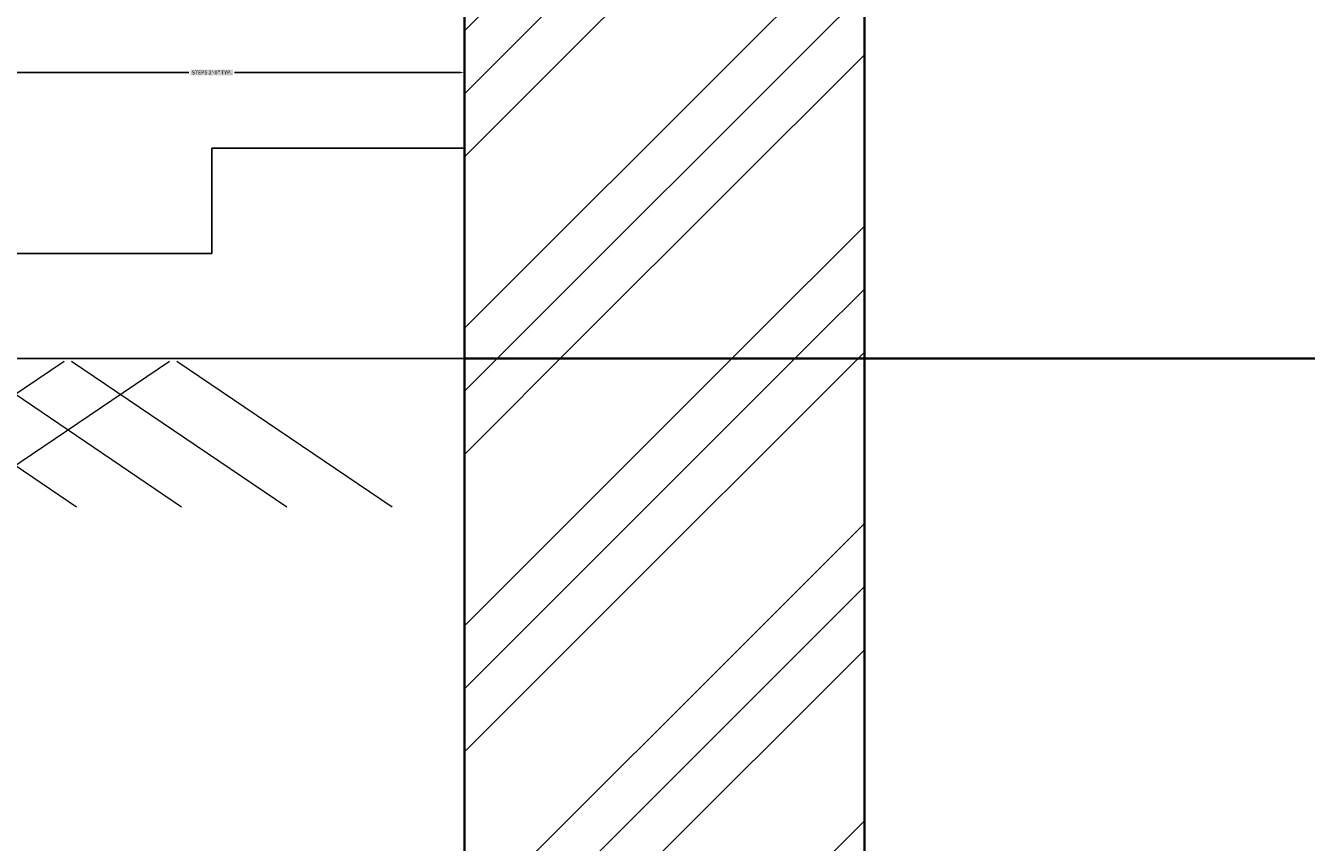
# Model space of a CAD drawing. Units: inches. Extents: x -128 to 854, y -395 to 398.
# Tile 8 of 61: x -77 to -16, y -321 to -282. Entities that reach past the tile are written whole.
import ezdxf

# ---------------------------------------------------------------- set-up
doc = ezdxf.new("R2010")
doc.units = ezdxf.units.IN
doc.header["$MEASUREMENT"] = 0
for name, color, linetype, lineweight in [('A-ANNO-DIMS', 2, 'Continuous', 18), ('A-FLOR-STRS', 7, 'Continuous', 25), ('A-SECT', 220, 'Continuous', 35), ('A-SECT-PATT', 8, 'Continuous', 13), ('C-GRAD', 7, 'Continuous', 25), ('C-GRAD-PATT', 8, 'Continuous', 13), ('S-FNDN', 2, 'Continuous', 35)]:
    doc.layers.add(name, color=color, linetype=linetype, lineweight=lineweight)
doc.styles.get("Standard").update_dxf_attribs({"font": 'arial.ttf'})
doc.dimstyles.get("Standard").update_dxf_attribs({"dimtxt": 0.18, "dimasz": 0.18, "dimexe": 0.18, "dimexo": 0.0625, "dimgap": 0.09, "dimtad": 0, "dimtih": 1, "dimtoh": 1, "dimdec": 1, "dimzin": 0, "dimdsep": 46, "dimlunit": 4, "dimtxsty": 'Standard', "dimcen": 0.09, "dimclrd": 1, "dimclre": 2, "dimclrt": 6, "dimadec": 0, "dimazin": 0, "dimtfac": 1, "dimtdec": 1, "dimtofl": 0, "dimtmove": 0, "dimatfit": 3, "dimfxl": 1, "dimtfill": 2, "dimtfillclr": 3, "dimtolj": 1, "dimtzin": 0, "dimarcsym": 0})

# ---------------------------------------------------------------- blocks, each defined once
blk = doc.blocks.new('ENTRY-STEPS-SECTION')
for p, q in [((12, 5), (12, 10)), ((12, 10), (24, 10)), ((0, 0), (0, 5)), ((0, 5), (12, 5)), ((24, 0), (0, 0))]:
    blk.add_line(p, q)
blk = doc.blocks.new('*D89')
at = {"layer": 'A-ANNO-DIMS', "color": 2, "lineweight": -2, "transparency": 16777216}
for p, q in [((-80.161, -287.957), (-80.161, -284.239)), ((-56.161, -287.957), (-56.161, -284.239))]:
    blk.add_line(p, q, dxfattribs=at)
at = {"layer": 'A-ANNO-DIMS', "color": 1, "lineweight": -2, "transparency": 16777216}
for p, q in [((-79.981, -284.419), (-69.246, -284.419)), ((-56.341, -284.419), (-67.076, -284.419))]:
    blk.add_line(p, q, dxfattribs=at)
at = {"layer": 'A-ANNO-DIMS', "color": 1, "transparency": 16777216}
for points in [[(-79.981, -284.389), (-79.981, -284.449), (-80.161, -284.419)], [(-56.341, -284.389), (-56.341, -284.449), (-56.161, -284.419)]]:
    blk.add_solid(points, dxfattribs=at)
at = {"layer": 'Defpoints', "color": 0, "transparency": 16777216}
for p in [(-56.161, -284.419), (-80.161, -288.019), (-56.161, -288.019)]:
    blk.add_point(p, dxfattribs=at)
at = {"layer": 'A-ANNO-DIMS', "color": 6, "transparency": 16777216, "insert": (-68.161, -284.419), "char_height": 0.18, "attachment_point": 5, "bg_fill": 1, "box_fill_scale": 1.25, "bg_fill_color": 3, "bg_fill_transparency": 0}
blk.add_mtext('\\A1;STEPS 2\'-0" TYP.', dxfattribs=at)
blk = doc.blocks.new('*D121')
at = {"layer": 'A-ANNO-DIMS', "color": 2, "lineweight": -2, "transparency": 16777216}
for p, q in [((-56.223, -298.019), (-128.041, -298.019)), ((-76.223, -358.019), (-128.041, -358.019))]:
    blk.add_line(p, q, dxfattribs=at)
at = {"layer": 'A-ANNO-DIMS', "color": 1, "lineweight": -2, "transparency": 16777216}
for p, q in [((-127.861, -298.199), (-127.861, -327.837)), ((-127.861, -357.839), (-127.861, -328.201))]:
    blk.add_line(p, q, dxfattribs=at)
at = {"layer": 'A-ANNO-DIMS', "color": 1, "transparency": 16777216}
for points in [[(-127.891, -298.199), (-127.831, -298.199), (-127.861, -298.019)], [(-127.891, -357.839), (-127.831, -357.839), (-127.861, -358.019)]]:
    blk.add_solid(points, dxfattribs=at)
at = {"layer": 'Defpoints', "color": 0, "transparency": 16777216}
for p in [(-56.161, -298.019), (-127.861, -358.019), (-76.161, -358.019)]:
    blk.add_point(p, dxfattribs=at)
at = {"layer": 'A-ANNO-DIMS', "color": 6, "transparency": 16777216, "insert": (-127.861, -328.019), "char_height": 0.18, "attachment_point": 5, "bg_fill": 1, "box_fill_scale": 1.25, "bg_fill_color": 3, "bg_fill_transparency": 0}
blk.add_mtext('\\A1;5\'-0"', dxfattribs=at)
blk = doc.blocks.new('*D125')
at = {"layer": 'A-ANNO-DIMS', "color": 2, "lineweight": -2, "transparency": 16777216}
for p, q in [((-37.161, -298.082), (-37.161, -381.899)), ((22.811, -298.082), (22.811, -381.899))]:
    blk.add_line(p, q, dxfattribs=at)
at = {"layer": 'A-ANNO-DIMS', "color": 1, "lineweight": -2, "transparency": 16777216}
for p, q in [((-36.981, -381.719), (-7.504, -381.719)), ((22.631, -381.719), (-6.846, -381.719))]:
    blk.add_line(p, q, dxfattribs=at)
at = {"layer": 'A-ANNO-DIMS', "color": 1, "transparency": 16777216}
for points in [[(-36.981, -381.689), (-36.981, -381.749), (-37.161, -381.719)], [(22.631, -381.689), (22.631, -381.749), (22.811, -381.719)]]:
    blk.add_solid(points, dxfattribs=at)
at = {"layer": 'Defpoints', "color": 0, "transparency": 16777216}
for p in [(-37.161, -298.019), (22.811, -298.019), (22.811, -381.719)]:
    blk.add_point(p, dxfattribs=at)
at = {"layer": 'A-ANNO-DIMS', "color": 6, "transparency": 16777216, "insert": (-7.175, -381.719), "char_height": 0.18, "attachment_point": 5, "bg_fill": 1, "box_fill_scale": 1.25, "bg_fill_color": 3, "bg_fill_transparency": 0}
blk.add_mtext('\\A1;5\'-0"', dxfattribs=at)

msp = doc.modelspace()

# ---------------------------------------------------------------- hatches: boundary and pattern name
at = {"layer": 'A-SECT-PATT'}
h = msp.add_hatch(dxfattribs=at)
h.set_pattern_fill('GOST_GROUND', color=256)
h.set_pattern_definition([(45, (0, 0), (14.14214, -9e-16), [20]), (45, (3, 0), (14.14214, -9e-16), [20]), (45, (6, 0), (14.14214, -9e-16), [20])])
h.paths.add_polyline_path([(-27.161, -322.019), (-37.161, -322.019), (-37.161, -298.019), (-56.161, -298.019), (-56.161, -322.019), (-66.161, -322.019), (-66.161, -346.019), (-27.161, -346.019)])
h.paths.add_polyline_path([(170.839, -322.019), (160.839, -322.019), (160.839, -298.019), (155.839, -298.019), (141.839, -298.019), (141.839, -322.019), (131.839, -322.019), (131.839, -346.019), (170.839, -346.019)])
h.paths.add_polyline_path([(327.839, -322.019), (317.839, -322.019), (317.839, -298.019), (312.839, -298.019), (298.839, -298.019), (298.839, -322.019), (288.839, -322.019), (288.839, -346.019), (327.839, -346.019)])
h.paths.add_polyline_path([(-37.161, -274.019), (-56.161, -274.019), (-56.161, -298.019), (-37.161, -298.019)])
h.paths.add_polyline_path([(-37.161, -207.019), (-56.161, -207.019), (-56.161, -226.019), (-37.161, -226.019)])
h.paths.add_polyline_path([(160.839, -274.019), (141.839, -274.019), (141.839, -298.019), (155.839, -298.019), (160.839, -298.019)])
at = {"layer": 'C-GRAD-PATT'}
h = msp.add_hatch(dxfattribs=at)
h.set_pattern_fill('ANSI31', color=256, scale=22.43157, angle=349.1104, style=0)
h.paths.add_polyline_path([(-94.192, -298.137), (-69.212, -298.137), (-79.439, -305.063), (-104.419, -305.063)])
h = msp.add_hatch(dxfattribs=at)
h.set_pattern_fill('ANSI31', color=256, scale=22.43157, angle=100.8896, style=0)
h.paths.add_polyline_path([(-94.192, -298.137), (-69.212, -298.137), (-58.986, -305.063), (-83.966, -305.063)])

# ---------------------------------------------------------------- linework, layer by layer
at = {"layer": 'A-SECT'}
for p, q in [((-56.161, -298.019), (-56.161, -178.019)), ((-37.161, -298.019), (-37.161, -178.019)), ((-56.161, -298.019), (312.839, -298.019)), ((-56.161, -298.019), (-37.161, -298.019))]:
    msp.add_line(p, q, dxfattribs=at)
at = {"layer": 'C-GRAD'}
msp.add_line((-56.161, -298.019), (-104.161, -298.019), dxfattribs=at)
at = {"layer": 'S-FNDN'}
for p, q in [((-51.161, -298.019), (-56.161, -298.019)), ((-56.161, -298.019), (-56.161, -322.019)), ((-42.161, -298.019), (-37.161, -298.019)), ((-37.161, -298.019), (-37.161, -322.019))]:
    msp.add_line(p, q, dxfattribs=at)

# ---------------------------------------------------------------- block references
at = {"layer": 'A-FLOR-STRS'}
msp.add_blockref('ENTRY-STEPS-SECTION', (-80.161, -298.019), dxfattribs=at)

# ---------------------------------------------------------------- dimensions: what is measured, and where the dimension line sits
at = {"layer": 'A-ANNO-DIMS'}
dim = msp.add_linear_dim(base=(-56.161, -284.419), p1=(-80.161, -288.019), p2=(-56.161, -288.019), text='STEPS <> TYP.', dimstyle='Standard', override={"dimdec": 1, "dimlfac": 1, "dimrnd": 0, "dimzin": 1, "dimdsep": 46, "dimlunit": 4, "dimfrac": 2}, dxfattribs=at)
dim.commit()
dim.dimension.update_dxf_attribs({"geometry": '*D89', "text_midpoint": (-68.161, -284.419)})
dim = msp.add_linear_dim(base=(-127.861, -358.019), p1=(-56.161, -298.019), p2=(-76.161, -358.019), angle=90, dimstyle='Standard', override={"dimdec": 1, "dimlfac": 1, "dimrnd": 0, "dimzin": 1, "dimdsep": 46, "dimlunit": 4, "dimfrac": 2}, dxfattribs=at)
dim.commit()
dim.dimension.update_dxf_attribs({"geometry": '*D121', "text_midpoint": (-127.861, -328.019)})
dim = msp.add_linear_dim(base=(22.811, -381.719), p1=(-37.161, -298.019), p2=(22.811, -298.019), dimstyle='Standard', override={"dimdec": 1, "dimlfac": 1, "dimrnd": 0, "dimzin": 1, "dimdsep": 46, "dimlunit": 4, "dimfrac": 2}, dxfattribs=at)
dim.commit()
dim.dimension.update_dxf_attribs({"geometry": '*D125', "text_midpoint": (-7.175, -381.719)})

doc.saveas('drawing.dxf')
